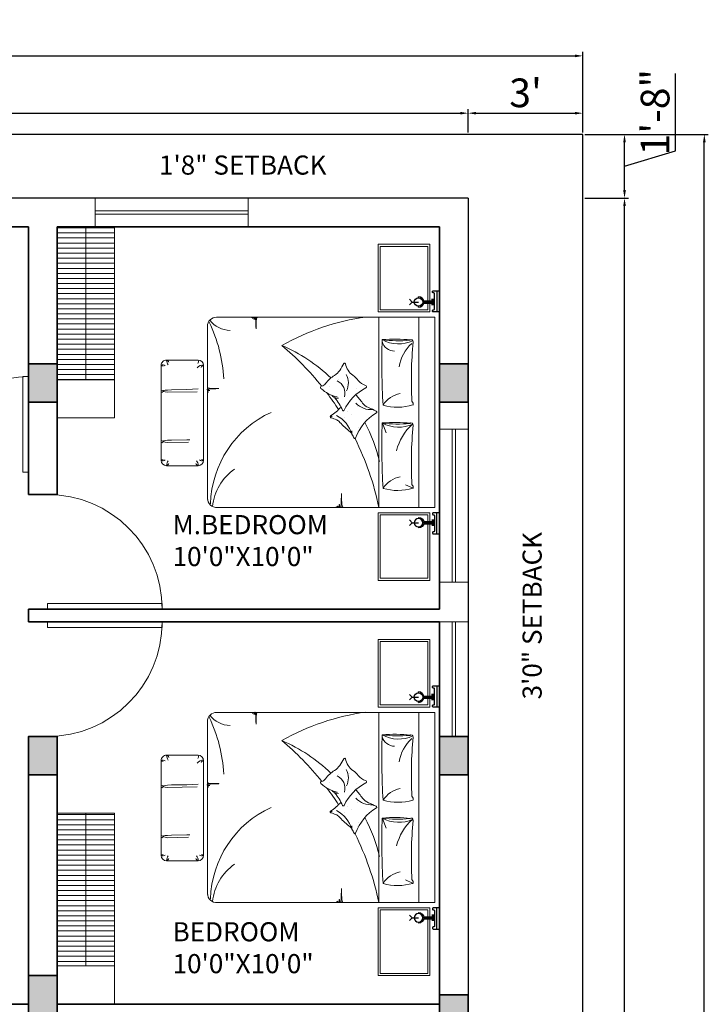
# Model space of a CAD drawing. Units: inches. Extents: x 3321 to 5237, y 11 to 1752.
# Tile 23 of 43: x 4325 to 4541, y 1434 to 1743. Entities that reach past the tile are written whole.
import ezdxf

# ---------------------------------------------------------------- set-up
doc = ezdxf.new("R2010")
doc.units = ezdxf.units.IN
for name, color, linetype, lineweight in [('A-ANNO-DIMS', 2, 'Continuous', 18), ('A-ANNO-TEXT', 7, 'Continuous', 18), ('A-AREA-IDEN', 7, 'Continuous', 18), ('A-COLS', 1, 'Continuous', 35), ('A-DOOR', 4, 'Continuous', 18), ('A-FLOR-CASE', 8, 'Continuous', 18), ('A-FLOR-CASE-PATT', 8, 'Continuous', 13), ('A-FLOR-EDGE', 7, 'Continuous', 25), ('A-GLAZ', 5, 'Continuous', 18), ('A-WALL', 7, 'Continuous', 35), ('C-PROP', 7, 'Continuous', 30), ('FUR', 42, 'Continuous', 18)]:
    doc.layers.add(name, color=color, linetype=linetype, lineweight=lineweight)
for name, color, linetype in [('CEIL', 4, 'Continuous'), ('ELEC', 4, 'Continuous'), ('wood', 26, 'Continuous')]:
    doc.layers.add(name, color=color, linetype=linetype)
doc.styles.get("Standard").update_dxf_attribs({"font": 'arial.ttf'})
doc.dimstyles.new('ISO-25', dxfattribs={"dimtxt": 9, "dimasz": 2.5, "dimexe": 1.25, "dimexo": 0.625, "dimtad": 1, "dimdec": 1, "dimlunit": 3, "dimtxsty": 'Standard', "dimcen": 2.5, "dimclrd": 4, "dimclre": 4, "dimclrt": 256, "dimadec": 0, "dimazin": 0, "dimtfac": 1, "dimtdec": 1, "dimtmove": 0, "dimatfit": 3, "dimfxl": 1, "dimarcsym": 0})
pattern_1 = [(180, (-735.7874, -1e-13), (-1e-16, -1.5875), [])]

# ---------------------------------------------------------------- blocks, each defined once
blk = doc.blocks.new('*U4')
for p, q in [((0, 0), (0, -6)), ((-36, 0), (-36, -6))]:
    blk.add_line(p, q)
blk.add_lwpolyline([(0, 0), (0, 36), (-1.75, 36), (-1.75, 0)], close=True)
blk.add_arc((0, 0), 36, 90, 180)
blk = doc.blocks.new('*U5')
for p, q in [((0, 0), (0, -6)), ((-30, 0), (-30, -6))]:
    blk.add_line(p, q)
blk.add_lwpolyline([(0, 0), (0, 30), (-1.75, 30), (-1.75, 0)], close=True)
blk.add_arc((0, 0), 30, 90, 180)
blk = doc.blocks.new('*D50')
at = {"layer": 'A-ANNO-DIMS', "color": 0, "lineweight": -2, "transparency": 16777216}
for p, q in [((4126.39, 1707.96), (4126.39, 1715.23)), ((4465.39, 1707.96), (4465.39, 1715.23)), ((4128.89, 1713.98), (4462.89, 1713.98))]:
    blk.add_line(p, q, dxfattribs=at)
at = {"layer": 'A-ANNO-DIMS', "color": 0, "transparency": 16777216}
for points in [[(4128.89, 1714.4), (4128.89, 1713.56), (4126.39, 1713.98)], [(4462.89, 1714.4), (4462.89, 1713.56), (4465.39, 1713.98)]]:
    blk.add_solid(points, dxfattribs=at)
at = {"layer": 'Defpoints', "color": 0, "transparency": 16777216}
for p in [(4465.39, 1713.98), (4126.39, 1707.34), (4465.39, 1707.34)]:
    blk.add_point(p, dxfattribs=at)
at = {"layer": 'A-ANNO-DIMS', "color": 0, "transparency": 16777216, "insert": (4295.89, 1719.2), "char_height": 9, "attachment_point": 5}
blk.add_mtext('28\'-3"', dxfattribs=at)
blk = doc.blocks.new('*D51')
at = {"layer": 'A-ANNO-DIMS', "color": 0, "lineweight": -2, "transparency": 16777216}
for p, q in [((4465.39, 1707.96), (4465.39, 1715.23)), ((4501.39, 1707.96), (4501.39, 1715.23)), ((4467.89, 1713.98), (4498.89, 1713.98))]:
    blk.add_line(p, q, dxfattribs=at)
at = {"layer": 'A-ANNO-DIMS', "color": 0, "transparency": 16777216}
for points in [[(4467.89, 1714.4), (4467.89, 1713.56), (4465.39, 1713.98)], [(4498.89, 1714.4), (4498.89, 1713.56), (4501.39, 1713.98)]]:
    blk.add_solid(points, dxfattribs=at)
at = {"layer": 'Defpoints', "color": 0, "transparency": 16777216}
for p in [(4501.39, 1713.98), (4465.39, 1707.34), (4501.39, 1707.34)]:
    blk.add_point(p, dxfattribs=at)
at = {"layer": 'A-ANNO-DIMS', "color": 0, "transparency": 16777216, "insert": (4483.39, 1719.2), "char_height": 9, "attachment_point": 5}
blk.add_mtext("3'", dxfattribs=at)
blk = doc.blocks.new('*D61')
at = {"layer": 'A-ANNO-DIMS', "color": 0, "lineweight": -2, "transparency": 16777216}
for p, q in [((4502.01, 1687.34), (4515.69, 1687.34)), ((4514.44, 1093.84), (4514.44, 1684.84)), ((4502.01, 1091.34), (4515.69, 1091.34))]:
    blk.add_line(p, q, dxfattribs=at)
at = {"layer": 'A-ANNO-DIMS', "color": 0, "transparency": 16777216}
for points in [[(4514.03, 1684.84), (4514.86, 1684.84), (4514.44, 1687.34)], [(4514.03, 1093.84), (4514.86, 1093.84), (4514.44, 1091.34)]]:
    blk.add_solid(points, dxfattribs=at)
at = {"layer": 'Defpoints', "color": 0, "transparency": 16777216}
for p in [(4501.39, 1687.34), (4514.44, 1687.34), (4501.39, 1091.34)]:
    blk.add_point(p, dxfattribs=at)
at = {"layer": 'A-ANNO-DIMS', "color": 0, "transparency": 16777216, "insert": (4509.22, 1389.34), "char_height": 9, "attachment_point": 5, "rotation": 90}
blk.add_mtext('49\'-8"', dxfattribs=at)
blk = doc.blocks.new('*D62')
at = {"layer": 'A-ANNO-DIMS', "color": 0, "lineweight": -2, "transparency": 16777216}
for p, q in [((4530.42, 1702.13), (4530.42, 1726.46)), ((4502.01, 1707.34), (4515.69, 1707.34)), ((4514.44, 1689.84), (4514.44, 1704.84)), ((4514.44, 1697.34), (4530.42, 1702.13)), ((4502.01, 1687.34), (4515.69, 1687.34))]:
    blk.add_line(p, q, dxfattribs=at)
at = {"layer": 'A-ANNO-DIMS', "color": 0, "transparency": 16777216}
for points in [[(4514.03, 1704.84), (4514.86, 1704.84), (4514.44, 1707.34)], [(4514.03, 1689.84), (4514.86, 1689.84), (4514.44, 1687.34)]]:
    blk.add_solid(points, dxfattribs=at)
at = {"layer": 'Defpoints', "color": 0, "transparency": 16777216}
for p in [(4501.39, 1707.34), (4514.44, 1707.34), (4501.39, 1687.34)]:
    blk.add_point(p, dxfattribs=at)
at = {"layer": 'A-ANNO-DIMS', "color": 0, "transparency": 16777216, "insert": (4525.2, 1714.29), "char_height": 9, "attachment_point": 5, "rotation": 90}
blk.add_mtext('1\'-8"', dxfattribs=at)
blk = doc.blocks.new('*D63')
at = {"layer": 'A-ANNO-DIMS', "color": 0, "lineweight": -2, "transparency": 16777216}
for p, q in [((4021.39, 1707.96), (4021.39, 1733.22)), ((4023.89, 1731.97), (4498.89, 1731.97)), ((4501.39, 1707.96), (4501.39, 1733.22))]:
    blk.add_line(p, q, dxfattribs=at)
at = {"layer": 'A-ANNO-DIMS', "color": 0, "transparency": 16777216}
for points in [[(4023.89, 1732.39), (4023.89, 1731.55), (4021.39, 1731.97)], [(4498.89, 1732.39), (4498.89, 1731.55), (4501.39, 1731.97)]]:
    blk.add_solid(points, dxfattribs=at)
at = {"layer": 'Defpoints', "color": 0, "transparency": 16777216}
for p in [(4501.39, 1731.97), (4021.39, 1707.34), (4501.39, 1707.34)]:
    blk.add_point(p, dxfattribs=at)
at = {"layer": 'A-ANNO-DIMS', "color": 0, "transparency": 16777216, "insert": (4261.39, 1737.19), "char_height": 9, "attachment_point": 5}
blk.add_mtext("40'", dxfattribs=at)
blk = doc.blocks.new('*D64')
at = {"layer": 'A-ANNO-DIMS', "color": 0, "lineweight": -2, "transparency": 16777216}
for p, q in [((4502.01, 1707.34), (4540.73, 1707.34)), ((4539.48, 989.84), (4539.48, 1704.84)), ((4502.01, 987.34), (4540.73, 987.34))]:
    blk.add_line(p, q, dxfattribs=at)
at = {"layer": 'A-ANNO-DIMS', "color": 0, "transparency": 16777216}
for points in [[(4539.06, 1704.84), (4539.9, 1704.84), (4539.48, 1707.34)], [(4539.06, 989.84), (4539.9, 989.84), (4539.48, 987.34)]]:
    blk.add_solid(points, dxfattribs=at)
at = {"layer": 'Defpoints', "color": 0, "transparency": 16777216}
for p in [(4501.39, 1707.34), (4539.48, 1707.34), (4501.39, 987.34)]:
    blk.add_point(p, dxfattribs=at)
at = {"layer": 'A-ANNO-DIMS', "color": 0, "transparency": 16777216, "insert": (4534.26, 1347.34), "char_height": 9, "attachment_point": 5, "rotation": 90}
blk.add_mtext("60'", dxfattribs=at)
blk = doc.blocks.new('*X127')
at = {"color": 0}
for p, q in [((3147.8, 8143.4), (3147.8, 8143.4)), ((3155.9, 8182.9), (3155.9, 8182.9)), ((3209.5, 8023.9), (3209.5, 8023.9)), ((3283, 8049.6), (3283, 8049.6)), ((3154.1, 7950.7), (3154.1, 7950.7)), ((3251.6, 7997), (3251.6, 7997))]:
    blk.add_line(p, q, dxfattribs=at)
blk = doc.blocks.new('*X126')
at = {"color": 0}
for p, q in [((3155.9, 8182.9), (3155.9, 8182.9)), ((3139.8, 7939.7), (3139.8, 7939.7))]:
    blk.add_line(p, q, dxfattribs=at)
blk = doc.blocks.new('*X125')
at = {"color": 0}
for p, q in [((3155.9, 8182.9), (3155.9, 8182.9)), ((3139.8, 7939.7), (3139.8, 7939.7))]:
    blk.add_line(p, q, dxfattribs=at)
blk = doc.blocks.new('*X124')
at = {"color": 0}
for p, q in [((3163, 7776.2), (3163, 7776.2)), ((3422.2, 7761.3), (3422.2, 7761.3)), ((3236.2, 7675.7), (3236.2, 7675.7)), ((3244.3, 7698.6), (3244.3, 7698.6)), ((3340.3, 7689.4), (3340.3, 7689.4))]:
    blk.add_line(p, q, dxfattribs=at)
blk = doc.blocks.new('BED1')
for p, q in [((0, -1000), (0, 800)), ((150, 800), (0, 800)), ((150, 800), (150, -1000)), ((2058.7, 800), (150, 800)), ((528, 800), (528, -1000)), ((211.8, 614.9), (277.5, 585.4)), ((2537.2, 404.9), (2237.2, 404.9)), ((2187.2, 354.9), (2187.2, -545.1)), ((2587.2, -545.1), (2587.2, 354.9)), ((2582, 188.1), (2565.4, 174.8)), ((2566.3, 178.5), (2565.2, 177.4)), ((2565.4, 174.8), (2585.7, 165.4)), ((2566.3, -296.8), (2565.2, -297.9)), ((2582, -287.1), (2565.4, -300.5)), ((2565.4, -300.5), (2585.7, -309.9)), ((2237.2, -595.1), (2537.2, -595.1)), ((150, -1000), (0, -1000)), ((150, -1000), (2063.5, -1000))]:
    blk.add_line(p, q)
for points in [[(934, 797.9), (930.9, 797.7), (928.3, 797.4), (926.3, 796.9), (924.9, 796.3), (923.8, 795.6), (923.1, 794.8), (922.7, 793.8), (922.5, 792.7), (922.4, 791.5), (922.5, 790.3), (922.6, 789.2), (922.6, 788.3), (922.6, 787.6), (922.4, 787.3), (922, 787.4), (921.4, 787.9), (920.6, 788.9), (919.5, 790.2), (918.4, 791.6), (917.1, 793.1), (915.9, 794.6), (914.6, 796), (913.3, 797.1), (912.2, 797.9), (911.1, 798.3), (910.1, 798.4), (909.2, 798), (908.3, 797.1), (907.5, 795.8), (906.8, 793.9), (906, 791.4), (905.4, 788.5), (904.8, 785.2), (904.2, 781.7), (903.7, 778.4), (903.2, 775.4), (902.8, 772.9), (902.5, 771.3), (902.3, 770.6), (902.1, 771.2), (902, 772.8), (901.8, 775.2), (901.7, 778.1), (901.5, 781.5), (901.2, 785), (900.8, 788.4), (900.2, 791.5), (899.5, 794.1), (898.6, 796.2), (897.6, 797.9), (896.5, 799.2), (895.3, 800), (894.1, 800.5), (893, 800.7), (891.9, 800.5), (890.9, 800.1), (890, 799), (889.1, 797.1), (888.3, 794), (887.6, 789.3), (886.9, 782.9), (886.2, 774.2), (885.5, 763.1), (884.8, 749.5), (884.2, 734.2), (883.6, 718.3), (883, 702.8), (882.5, 688.8), (882, 677.5), (881.7, 669.8), (881.5, 666.9), (881.3, 669.4), (881.3, 676.7), (881.3, 687.8), (881.2, 701.5), (881.1, 716.8), (880.8, 732.6), (880.2, 748), (879.4, 761.8), (878.3, 773.2), (876.9, 782.2), (875.1, 789.2), (872.9, 794.4), (870.3, 798), (869, 799)], [(2150, -913.5), (2150, 723.2)], [(494.7, 3.1), (458.9, 95.3)], [(2327.6, 182.3), (2530, 185.9), (2550.8, 181.9), (2561.7, 179), (2566, 176.7), (2566.9, 174.4), (2566.3, 171.9), (2562, 169.2), (2550.3, 166.5), (2527.7, 163.9), (2490.6, 161.8), (2345.5, 160.2), (2317.8, 158.5)], [(2149.7, -259.9), (2150, -268.4), (2150.1, -274.1), (2150.1, -278.1), (2150, -281.4), (2149.8, -284), (2149.5, -286.1), (2149.1, -287.8), (2148.7, -289), (2148.1, -289.9), (2147.4, -290.5), (2146.6, -290.8), (2145.6, -291), (2144.6, -291), (2143.6, -291), (2142.7, -290.9), (2141.9, -290.9), (2141.4, -290.9), (2141.1, -291), (2141.2, -291.4), (2141.7, -291.9), (2142.5, -292.6), (2143.5, -293.4), (2144.7, -294.4), (2146, -295.4), (2147.2, -296.5), (2148.4, -297.6), (2149.3, -298.6), (2150, -299.6), (2150.3, -300.5), (2150.4, -301.3), (2150, -302.1), (2149.3, -302.8), (2148.2, -303.5), (2146.6, -304.1), (2144.6, -304.7), (2142.1, -305.2), (2139.3, -305.7), (2136.5, -306.2), (2133.7, -306.6), (2131.2, -307), (2129.2, -307.3), (2127.8, -307.6), (2127.3, -307.8), (2127.7, -308), (2129, -308.1), (2131, -308.2), (2133.5, -308.3), (2136.3, -308.5), (2139.2, -308.7), (2142, -309), (2144.6, -309.5), (2146.8, -310.1), (2148.6, -310.9), (2150, -311.7), (2151, -312.7), (2151.7, -313.6), (2152.1, -314.6), (2152.3, -315.6), (2152.2, -316.5), (2151.8, -317.3), (2150.9, -318.1), (2149.3, -318.8), (2146.7, -319.4), (2142.8, -320), (2137.4, -320.6), (2130.2, -321.2), (2121, -321.8), (2109.7, -322.3), (2096.9, -322.9), (2083.6, -323.4), (2070.7, -323.9), (2059.1, -324.3), (2049.6, -324.7), (2043.2, -325), (2040.8, -325.2), (2042.9, -325.3), (2049, -325.3), (2058.2, -325.3), (2069.6, -325.4), (2082.3, -325.5), (2095.6, -325.8), (2108.4, -326.2), (2119.9, -326.8), (2129.4, -327.8), (2136.9, -329), (2142.7, -330.5), (2147, -332.3), (2150, -334.4), (2150.9, -335.6)], [(2246.5, -294.4), (2530, -289.4), (2550.8, -293.4), (2561.7, -296.3), (2566, -298.6), (2566.9, -300.8), (2566.3, -303.4), (2562, -306.1), (2550.3, -308.8), (2527.7, -311.3), (2490.6, -313.5), (2345.5, -315), (2238.6, -321.8)], [(1733.7, -998.3), (1731.1, -998.1), (1729, -997.8), (1727.4, -997.4), (1726.1, -997), (1725.2, -996.4), (1724.7, -995.7), (1724.3, -994.8), (1724.1, -993.9), (1724.1, -992.9), (1724.1, -991.9), (1724.2, -991), (1724.2, -990.2), (1724.2, -989.7), (1724.1, -989.4), (1723.8, -989.5), (1723.2, -990), (1722.5, -990.8), (1721.7, -991.8), (1720.7, -993), (1719.7, -994.3), (1718.6, -995.5), (1717.5, -996.6), (1716.5, -997.6), (1715.5, -998.3), (1714.6, -998.6), (1713.8, -998.6), (1713, -998.3), (1712.3, -997.6), (1711.7, -996.5), (1711, -994.9), (1710.4, -992.9), (1709.9, -990.4), (1709.4, -987.6), (1708.9, -984.8), (1708.5, -982), (1708.1, -979.5), (1707.8, -977.4), (1707.5, -976.1), (1707.3, -975.5), (1707.1, -976), (1707, -977.3), (1706.9, -979.3), (1706.8, -981.8), (1706.7, -984.6), (1706.4, -987.5), (1706.1, -990.3), (1705.6, -992.9), (1705, -995.1), (1704.2, -996.9), (1703.4, -998.3), (1702.4, -999.3), (1701.5, -1000), (1700.5, -1000.4), (1699.6, -1000.6), (1698.7, -1000.4), (1697.8, -1000.1), (1697, -999.2), (1696.3, -997.6), (1695.7, -995), (1695.1, -991.1), (1694.5, -985.7), (1693.9, -978.5), (1693.3, -969.3), (1692.8, -957.9), (1692.2, -945.2), (1691.7, -931.9), (1691.2, -919), (1690.8, -907.4), (1690.4, -897.9), (1690.1, -891.5), (1689.9, -889.1), (1689.8, -891.2), (1689.8, -897.3), (1689.8, -906.5), (1689.7, -917.9), (1689.6, -930.6), (1689.4, -943.8), (1688.9, -956.6), (1688.3, -968.1), (1687.3, -977.6), (1686.1, -985.2), (1684.6, -991), (1682.8, -995.3), (1680.7, -998.3), (1679.6, -999.2)]]:
    blk.add_lwpolyline(points)
for points in [[(205.5, 619.6, 0.267769), (215.1, 582.4, -0.037739), (204.3, 21.8, 0.684696), (236.7, 5.5, -0.060702), (497.2, 0.1, -0.046649), (225.9, 3.1, -1.318436)], [(489.2, 619.6, 0.144019), (207.6, 617.9, 0.248643)], [(497.2, 0.1, 0.021276), (489.2, 619.6, -0.206383), (326.6, 509.4, 0.237198)], [(211.8, 12.8, 0.143972), (361.6, 262.9, 1.292232)], [(886.4, -150, -0.069098), (985, -66.5, 0.658965), (982.1, -48.7, -0.049789), (927.4, -29, -0.103757), (896.6, -5.4, 0.055725), (800.9, 83.3, -0.11866), (782.7, 104.9, 0.016811), (761.6, 143.9, 0.70791), (748.3, 144, -0.16964), (551.9, -96.6, 0.664036), (554, -110.7, 0.023706), (627, -144.7, -0.134834), (683.2, -188, 0.012748), (746.3, -267.4)], [(205.5, -168.2, 0.267769), (215.1, -205.4, -0.037739), (204.3, -766, 0.684696), (236.7, -782.3, -0.060702), (497.2, -787.7, -0.046649), (225.9, -784.7, -1.318436)], [(489.2, -168.2, 0.144019), (207.6, -169.9, 0.248643)], [(497.2, -787.7, 0.021276), (489.2, -168.2, -0.206383), (326.6, -278.4, 0.237198)], [(969.1, -259.1, 0.263265), (936.3, -236.9, -0.026108), (909.2, -233.2, 0.027613), (945.1, -234.2, -0.089259), (872.7, -120, 0.662242), (857.6, -119.3, -0.162037), (651.8, -332.7, 0.676499), (654, -354.5, -0.160513), (722.9, -401.5, 0.07473), (773.5, -450.3, -0.187721), (845.5, -559.9, 0.70791), (858.8, -561.4, -0.010003), (898.6, -497.3, -0.113819), (947.3, -450.2, 0.099539), (1032.5, -372.4, -0.173425), (1070.9, -346.4, 0.589988), (1076.2, -326.1, 0.137312), (923.9, -245.9, 0.137312)], [(1446, -733.4, -0.095039), (652.8, -1001.7)]]:
    blk.add_lwpolyline(points, format="xyb")
for centre, radius, start, end in [((3208.8, 1363.3), 2739.4, 191.86791, 206.32469), ((1138.6, 793.9), 983.2, 294.60777, 358.30329), ((1608.1, 842.5), 496.3, 305.19014, 354.02057), ((2062.7, 713.7), 86.5, 0, 93.53765), ((2237.2, 354.9), 50, 90, 180), ((2321.1, 409.7), 84.5, 185.61958, 217.13957), ((2227.5, 373.5), 32.8, 17.83305, 72.80048), ((2546.9, 373.5), 32.8, 107.19952, 162.16695), ((2453.3, 409.7), 84.5, 322.86043, 354.38042), ((2537.2, 354.9), 50, 0, 90), ((2098.7, 754.7), 1625, 193.90497, 207.81692), ((2201.9, 323.3), 34.8, 50.8413, 114.9586), ((2212.2, 381.5), 36.5, 226.80948, 258.3841), ((2572.5, 323.3), 34.8, 65.0414, 129.1587), ((2562.2, 381.5), 36.5, 281.6159, 313.19052), ((751.8, 88.7), 34.9, 336.83517, 27.72181), ((684.2, 86), 100.3, 353.675, 10.88198), ((1074.1, 198.8), 306.1, 197.86019, 241.51221), ((341.4, -277.7), 318.5, 60.71255, 115.00895), ((983.7, -79.5), 20.8, 73.79673, 130.45661), ((978.5, -68.6), 14.3, 39.7097, 85.9506), ((602.5, -324), 198.6, 43.20348, 95.05559), ((3208.8, 1363.3), 2739.4, 212.93136, 216.95099), ((981.1, -281.8), 131.1, 164.0372, 243.45361), ((980, -379), 163.4, 152.61037, 209.36102), ((3208.8, 1363.3), 2739.4, 218.63292, 229.94485), ((2098.7, 754.7), 1625, 226.58872, 246.3156), ((3402.5, -342.9), 1408.5, 182.99169, 205.68187), ((-34.4, -471.2), 376.5, 312.01178, 350.96348), ((2178, -513.5), 33, 286.18268, 338.13858), ((2237.2, -545.1), 50, 180, 270), ((2188.1, -476.2), 73, 269.45125, 322.80265), ((2453.3, -600), 84.5, 5.61958, 37.13957), ((2537.2, -545.1), 50, 270, 0), ((2572.5, -513.6), 34.8, 230.8413, 294.9586), ((2562.2, -571.8), 36.5, 46.80948, 78.3841), ((2271.1, -580.9), 35.8, 148.90546, 197.55407), ((2546.9, -563.8), 32.8, 197.83305, 252.80048), ((375.7, -807.4), 128.2, 17.40732, 88.51286), ((341.4, -1065.5), 318.5, 60.71255, 115.00895), ((1929.1, -1126), 250.5, 37.85533, 88.44053), ((2063.5, -913.5), 86.5, 270, 0)]:
    blk.add_arc(centre, radius, start, end)
for name in ['*X126', '*X125', '*X127', '*X124']:
    blk.add_blockref(name, (-2425.3, -8101.4))
blk = doc.blocks.new('APLIQ')
at = {"layer": 'ELEC'}
for p, q in [((0, 0.2), (-0.0261, 0.2261)), ((0, 0.2), (0.0261, 0.2261)), ((0, 0.2), (0, 0.14)), ((-0.05, 0.14), (-0.04, 0.14)), ((0.04, 0.14), (0.05, 0.14)), ((-0.03, 0.01), (0.03, 0.01)), ((-0.03, 0), (0.03, 0)), ((-0.01, 0.09), (-0.01, 0.01)), ((0, 0.09), (0, 0)), ((0.01, 0.09), (0.01, 0.01))]:
    blk.add_line(p, q, dxfattribs=at)
blk.add_circle((0, 0.14), 0.04, dxfattribs=at)
blk.add_arc((0, 0.14), 0.05, 180, 0, dxfattribs=at)
blk = doc.blocks.new('A$C68AE1801')
at = {"layer": 'FUR'}
for points in [[(2.5416, 3.18), (2.5416, 2.54), (2.0516, 2.54), (2.0516, 3.18)], [(2.5216, 3.16), (2.5216, 2.56), (2.0716, 2.56), (2.0716, 3.16)], [(2.5416, 0), (2.5416, 0.64), (2.0516, 0.64), (2.0516, 0)], [(2.5216, 0.02), (2.5216, 0.62), (2.0716, 0.62), (2.0716, 0.02)]]:
    blk.add_lwpolyline(points, close=True, dxfattribs=at)
at = {"layer": 'wood'}
for p, q in [((2.6057, 2.74), (2.6057, 2.54)), ((2.6057, 0.44), (2.6057, 0.64))]:
    blk.add_line(p, q, dxfattribs=at)
for points in [[(2.5657, 2.728), (2.5657, 2.732, -0.414214), (2.5737, 2.74), (2.6321, 2.74), (2.6321, 2.54), (2.5737, 2.54, -0.414214), (2.5657, 2.548), (2.5657, 2.552, -0.414214), (2.5737, 2.56), (2.5777, 2.56, 0.414214), (2.5857, 2.568), (2.5857, 2.712, 0.414214), (2.5777, 2.72), (2.5737, 2.72, -0.414214)], [(2.5657, 0.452), (2.5657, 0.448, 0.414214), (2.5737, 0.44), (2.6321, 0.44), (2.6321, 0.64), (2.5737, 0.64, 0.414214), (2.5657, 0.632), (2.5657, 0.628, 0.414214), (2.5737, 0.62), (2.5777, 0.62, -0.414214), (2.5857, 0.612), (2.5857, 0.468, -0.414214), (2.5777, 0.46), (2.5737, 0.46, 0.414214)]]:
    blk.add_lwpolyline(points, format="xyb", close=True, dxfattribs=at)
at = {"layer": 'CEIL', "rotation": 90}
blk.add_blockref('APLIQ', (2.5736, 2.634), dxfattribs=at)
at = {"layer": 'CEIL', "xscale": -1, "rotation": 90}
blk.add_blockref('APLIQ', (2.5736, 0.546), dxfattribs=at)
at = {"layer": 'FUR', "xscale": 0.001, "yscale": 0.001, "zscale": 0.001, "rotation": 180}
blk.add_blockref('BED1', (2.5872, 1.49), dxfattribs=at)
blk = doc.blocks.new('COL-9X18-IN')
h = blk.add_hatch(color=256)
h.dxf.hatch_style = 1
h.paths.add_polyline_path([(9, 18), (0, 18), (0, 0), (9, 0)])
blk.add_lwpolyline([(0, 0), (9, 0), (9, 18), (0, 18)], close=True)
blk = doc.blocks.new('COL-9X12-FURN-PLAN')
h = blk.add_hatch(color=256)
h.dxf.hatch_style = 1
h.paths.add_polyline_path([(0, 12), (0, 0), (9, 0), (9, 12)])
blk.add_lwpolyline([(0, 0), (9, 0), (9, 12), (0, 12)], close=True)
blk = doc.blocks.new('WIN-48IN-9IN-WALL')
for p, q in [((0, 0), (0, 9)), ((48, 0), (48, 9)), ((0, 5), (48, 5)), ((0, 4), (48, 4))]:
    blk.add_line(p, q)
blk = doc.blocks.new('WIN-36IN-9IN-WALL')
for p, q in [((9, 36), (0, 36)), ((4, 36), (4, 0)), ((5, 36), (5, 0)), ((9, 0), (0, 0))]:
    blk.add_line(p, q)
blk = doc.blocks.new('PROPERTY-40X60FT')
for p, q in [((0, 720), (0, 0)), ((0, 0), (480, 0))]:
    blk.add_line(p, q)

msp = doc.modelspace()

# ---------------------------------------------------------------- hatches: boundary and pattern name
at = {"layer": 'A-FLOR-CASE-PATT'}
h = msp.add_hatch(dxfattribs=at)
h.set_pattern_fill('ANSI31', color=256, scale=0.5, angle=135)
h.set_pattern_definition(pattern_1)
h.paths.add_polyline_path([(4354.39, 1630.34), (4354.39, 1678.34), (4336.39, 1678.34), (4336.39, 1630.34)])
h = msp.add_hatch(dxfattribs=at)
h.set_pattern_fill('ANSI31', color=256, scale=0.5, angle=135)
h.set_pattern_definition(pattern_1)
h.paths.add_polyline_path([(4354.39, 1494.34), (4336.39, 1494.34), (4336.39, 1446.34), (4354.39, 1446.34)])

# ---------------------------------------------------------------- linework, layer by layer
at = {"layer": 'A-FLOR-CASE'}
for p, q in [((4345.39, 1630.34), (4345.39, 1678.34)), ((4354.39, 1678.34), (4354.39, 1618.34)), ((4354.39, 1630.34), (4336.39, 1630.34)), ((4354.39, 1618.34), (4336.39, 1618.34)), ((4336.39, 1494.34), (4354.39, 1494.34)), ((4345.39, 1494.34), (4345.39, 1446.34)), ((4354.39, 1494.34), (4354.39, 1434.34)), ((4336.39, 1446.34), (4354.39, 1446.34))]:
    msp.add_line(p, q, dxfattribs=at)
at = {"layer": 'A-FLOR-EDGE'}
for q in [(4066.39, 1687.34), (4465.39, 1091.34)]:
    msp.add_line((4465.39, 1687.34), q, dxfattribs=at)
at = {"layer": 'A-WALL'}
for p, q in [((4327.39, 1678.34), (4278.39, 1678.34)), ((4327.39, 1678.34), (4327.39, 1594.34)), ((4336.39, 1678.34), (4336.39, 1594.34)), ((4456.39, 1678.34), (4336.39, 1678.34)), ((4456.39, 1678.34), (4456.39, 1558.34)), ((4336.39, 1594.34), (4327.39, 1594.34)), ((4456.39, 1558.34), (4327.39, 1558.34)), ((4327.39, 1558.34), (4327.39, 1554.34)), ((4327.39, 1554.34), (4456.39, 1554.34)), ((4456.39, 1554.34), (4456.39, 1434.34)), ((4327.39, 1518.34), (4336.39, 1518.34)), ((4327.39, 1518.34), (4327.39, 1443.34)), ((4336.39, 1518.34), (4336.39, 1434.34)), ((4135.39, 1434.34), (4327.39, 1434.34)), ((4336.39, 1434.34), (4456.39, 1434.34))]:
    msp.add_line(p, q, dxfattribs=at)

# ---------------------------------------------------------------- block references
at = {"layer": 'A-COLS'}
for p in [(4327.39, 1623.34), (4456.39, 1623.34), (4327.39, 1506.34), (4456.39, 1506.34), (4456.39, 1425.34)]:
    msp.add_blockref('COL-9X12-FURN-PLAN', p, dxfattribs=at)
at = {"layer": 'A-COLS', "rotation": 180}
msp.add_blockref('COL-9X18-IN', (4336.39, 1443.34), dxfattribs=at)
at = {"layer": 'A-DOOR'}
msp.add_blockref('*U5', (4327.39, 1601.34), dxfattribs=at)
at = {"layer": 'A-DOOR', "rotation": 270}
msp.add_blockref('*U4', (4333.39, 1558.34), dxfattribs=at)
at = {"layer": 'A-DOOR', "xscale": -1, "rotation": 270}
msp.add_blockref('*U4', (4333.39, 1554.34), dxfattribs=at)
at = {"layer": 'A-GLAZ'}
msp.add_blockref('WIN-48IN-9IN-WALL', (4348.36, 1678.34), dxfattribs=at)
for name, p, rotation in [('WIN-48IN-9IN-WALL', (4465.39, 1566.84), 89.99999999999824), ('WIN-36IN-9IN-WALL', (4465.39, 1554.34), 180)]:
    msp.add_blockref(name, p, dxfattribs=dict(at, rotation=rotation))
at = {"layer": 'C-PROP', "rotation": 180}
msp.add_blockref('PROPERTY-40X60FT', (4501.39, 1707.34), dxfattribs=at)
at = {"layer": 'FUR', "xscale": 33.17188472218209, "yscale": 33.17188472218209, "zscale": 33.17188472218209}
for p in [(4369.07, 1567.35), (4369.07, 1443.35)]:
    msp.add_blockref('A$C68AE1801', p, dxfattribs=at)

# ---------------------------------------------------------------- texts
at = {"layer": 'A-ANNO-TEXT', "insert": (4368.37, 1700.7), "char_height": 6, "attachment_point": 1}
msp.add_mtext_dynamic_manual_height_columns('1\'8" SETBACK', width=97.3114, gutter_width=25, heights=[0], dxfattribs=at)
at = {"layer": 'A-ANNO-TEXT', "insert": (4482.45, 1530.01), "char_height": 6, "attachment_point": 1, "rotation": 90}
msp.add_mtext_dynamic_manual_height_columns('3\'0" SETBACK', width=97.3114, gutter_width=25, heights=[0], dxfattribs=at)
at = {"layer": 'A-AREA-IDEN', "char_height": 6, "attachment_point": 1}
for s, insert in [('M.BEDROOM\\P10\'0"X10\'0"', (4372.64, 1587.85)), ('BEDROOM\\P10\'0"X10\'0"', (4372.64, 1460.08))]:
    msp.add_mtext_dynamic_manual_height_columns(s, width=97.3114, gutter_width=25, heights=[0], dxfattribs=dict(at, insert=insert))

# ---------------------------------------------------------------- dimensions: what is measured, and where the dimension line sits
at = {"layer": 'A-ANNO-DIMS'}
for base, p1, p2, override, picture, middle in [((4501.39, 1731.97), (4021.39, 1707.34), (4501.39, 1707.34), {"dimclrd": 0, "dimclre": 0, "dimclrt": 0}, '*D63', (4261.39, 1737.19)), ((4465.39, 1713.98), (4126.39, 1707.34), (4465.39, 1707.34), {"dimclrd": 0, "dimclre": 0, "dimclrt": 0, "dimtmove": 1}, '*D50', (4295.89, 1719.2)), ((4501.39, 1713.98), (4465.39, 1707.34), (4501.39, 1707.34), {"dimclrd": 0, "dimclre": 0, "dimclrt": 0, "dimtmove": 1}, '*D51', (4483.39, 1719.2))]:
    dim = msp.add_linear_dim(base=base, p1=p1, p2=p2, dimstyle='ISO-25', override=override, dxfattribs=at)
    dim.commit()
    dim.dimension.update_dxf_attribs({"geometry": picture, "text_midpoint": middle})
for base, p1, p2, angle, override, picture, middle in [((4514.44, 1707.34), (4501.39, 1687.34), (4501.39, 1707.34), 90, {"dimclrd": 0, "dimclre": 0, "dimclrt": 0, "dimtmove": 1}, '*D62', (4525.2, 1702.76)), ((4539.48, 1707.34), (4501.39, 987.34), (4501.39, 1707.34), 270, {"dimclrd": 0, "dimclre": 0, "dimclrt": 0}, '*D64', (4534.26, 1347.34)), ((4514.44, 1687.34), (4501.39, 1091.34), (4501.39, 1687.34), 90, {"dimclrd": 0, "dimclre": 0, "dimclrt": 0, "dimtmove": 1}, '*D61', (4509.22, 1389.34))]:
    dim = msp.add_linear_dim(base=base, p1=p1, p2=p2, angle=angle, dimstyle='ISO-25', override=override, dxfattribs=at)
    dim.commit()
    dim.dimension.update_dxf_attribs({"geometry": picture, "text_midpoint": middle})

doc.saveas('drawing.dxf')
